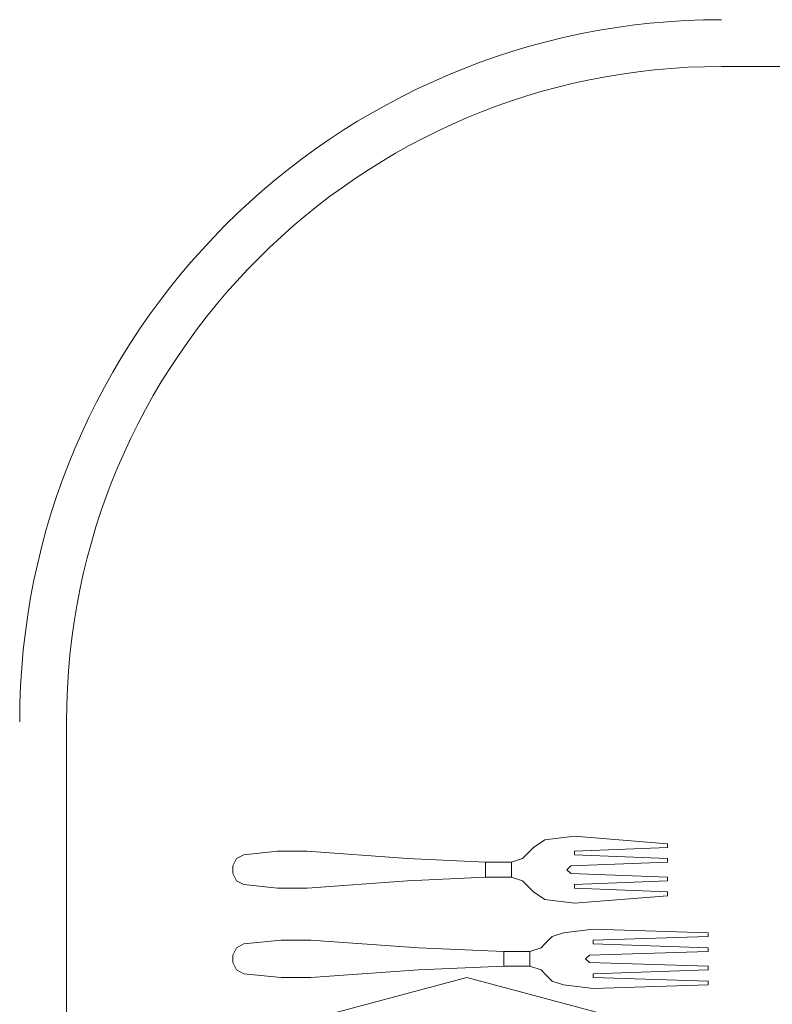
# Model space of a CAD drawing. Units: inches. Extents: x 375 to 1122, y 27 to 1069.
# Tile 125 of 155: x 705.14 to 717.62, y 900.21 to 916.52. Entities that reach past the tile are written whole.
import ezdxf

# ---------------------------------------------------------------- set-up
doc = ezdxf.new("R2010")
doc.units = ezdxf.units.IN
doc.layers.add('A-ANNO-DIMS', color=2, linetype='Continuous', lineweight=18)
doc.layers.add('Furniture', color=30, linetype='Continuous', lineweight=18)
doc.styles.get("Standard").update_dxf_attribs({"font": 'arial.ttf'})
doc.dimstyles.new('ISO-25', dxfattribs={"dimtxt": 12, "dimasz": 2.5, "dimexe": 1.5, "dimexo": 1.5, "dimtad": 1, "dimdec": 1, "dimlunit": 3, "dimtxsty": 'Standard', "dimblk": 'ARCHTICK', "dimcen": 2.5, "dimadec": 0, "dimazin": 0, "dimtfac": 1, "dimtdec": 1, "dimtmove": 0, "dimatfit": 3, "dimfxl": 1.5, "dimfxlon": 1, "dimarcsym": 0})

# ---------------------------------------------------------------- blocks, each defined once
blk = doc.blocks.new('A$C403C54AD')
for p, q in [((0.56427, 0.79569, -0.0006), (0.56427, 1.26108, -0.0006)), ((0.92321, 0.73013, -0.02105), (0.92475, 0.72551, -0.02059)), ((0.92321, 0.73013, -0.02413), (0.92475, 0.72551, -0.02367)), ((0.88473, 0.72244, -0.02105), (0.88781, 0.71782, -0.02059)), ((0.88473, 0.72244, -0.02413), (0.88781, 0.71782, -0.02367)), ((0.83575, 0.52421, -0.0006), (1.99923, 0.52421, -0.0006))]:
    blk.add_line(p, q)
for radius in [0.29087, 0.27148]:
    blk.add_arc((0.83575, 0.79569, -0.0006), radius, 180, 270)
for points, invisible_edges in [([(0.92629, 0.74244, -0.02045), (0.92167, 0.74244, -0.02045), (0.92321, 0.79016, -0.01335), (0.92475, 0.79016, -0.01335)], 1), ([(0.92629, 0.74244, -0.02353), (0.92167, 0.74244, -0.02353), (0.92321, 0.79016, -0.01643), (0.92475, 0.79016, -0.01643)], 1), ([(0.93244, 0.74091, -0.0207), (0.92782, 0.74244, -0.02045), (0.92936, 0.79016, -0.01335), (0.9309, 0.79016, -0.01335)], 1), ([(0.93244, 0.74091, -0.02378), (0.92782, 0.74244, -0.02353), (0.92936, 0.79016, -0.01643), (0.9309, 0.79016, -0.01643)], 1), ([(0.94014, 0.74244, -0.02045), (0.93552, 0.74091, -0.0207), (0.93706, 0.79016, -0.01335), (0.9386, 0.79016, -0.01335)], 1), ([(0.94014, 0.74244, -0.02353), (0.93552, 0.74091, -0.02378), (0.93706, 0.79016, -0.01643), (0.9386, 0.79016, -0.01643)], 1), ([(0.94168, 0.74244, -0.02045), (0.9463, 0.74244, -0.02045), (0.94476, 0.79016, -0.01335), (0.94322, 0.79016, -0.01335)], 1), ([(0.94168, 0.74244, -0.02353), (0.9463, 0.74244, -0.02353), (0.94476, 0.79016, -0.01643), (0.94322, 0.79016, -0.01643)], 1), ([(0.88935, 0.73475, -0.02045), (0.88319, 0.73475, -0.02045), (0.88627, 0.77323, -0.01335), (0.88781, 0.77323, -0.01335)], 1), ([(0.88935, 0.73475, -0.02353), (0.88319, 0.73475, -0.02353), (0.88627, 0.77323, -0.01643), (0.88781, 0.77323, -0.01643)], 1), ([(0.8955, 0.73321, -0.0207), (0.89088, 0.73475, -0.02045), (0.89242, 0.77323, -0.01335), (0.89396, 0.77323, -0.01335)], 1), ([(0.8955, 0.73321, -0.02378), (0.89088, 0.73475, -0.02353), (0.89242, 0.77323, -0.01643), (0.89396, 0.77323, -0.01643)], 1), ([(0.9032, 0.73475, -0.02045), (0.89858, 0.73321, -0.0207), (0.90012, 0.77323, -0.01335), (0.90166, 0.77323, -0.01335)], 1), ([(0.9032, 0.73475, -0.02353), (0.89858, 0.73321, -0.02378), (0.90012, 0.77323, -0.01643), (0.90166, 0.77323, -0.01643)], 1), ([(0.90474, 0.73475, -0.02045), (0.91089, 0.73475, -0.02045), (0.90782, 0.77323, -0.01335), (0.90628, 0.77323, -0.01335)], 1), ([(0.90474, 0.73475, -0.02353), (0.91089, 0.73475, -0.02353), (0.90782, 0.77323, -0.01643), (0.90628, 0.77323, -0.01643)], 1), ([(0.92321, 0.73013, -0.02105), (0.92782, 0.74244, -0.02045), (0.92629, 0.74244, -0.02045), (0.92167, 0.74244, -0.02045)], 5), ([(0.92321, 0.73013, -0.02413), (0.92782, 0.74244, -0.02353), (0.92629, 0.74244, -0.02353), (0.92167, 0.74244, -0.02353)], 5), ([(0.92321, 0.73013, -0.02413), (0.92321, 0.73013, -0.02105), (0.92167, 0.74244, -0.02045), (0.92167, 0.74244, -0.02353)], 1), ([(0.92321, 0.73013, -0.02105), (0.93398, 0.73924, -0.02085), (0.93244, 0.74091, -0.0207), (0.92782, 0.74244, -0.02045)], 13), ([(0.92321, 0.73013, -0.02413), (0.93398, 0.73924, -0.02392), (0.93244, 0.74091, -0.02378), (0.92782, 0.74244, -0.02353)], 13), ([(0.94476, 0.73013, -0.02105), (0.93398, 0.73924, -0.02085), (0.93552, 0.74091, -0.0207), (0.94014, 0.74244, -0.02045)], 13), ([(0.94476, 0.73013, -0.02413), (0.93398, 0.73924, -0.02392), (0.93552, 0.74091, -0.02378), (0.94014, 0.74244, -0.02353)], 13), ([(0.94476, 0.73013, -0.02105), (0.94014, 0.74244, -0.02045), (0.94168, 0.74244, -0.02045), (0.9463, 0.74244, -0.02045)], 5), ([(0.94476, 0.73013, -0.02413), (0.94014, 0.74244, -0.02353), (0.94168, 0.74244, -0.02353), (0.9463, 0.74244, -0.02353)], 5), ([(0.94476, 0.73013, -0.02105), (0.94476, 0.73013, -0.02413), (0.9463, 0.74244, -0.02353), (0.9463, 0.74244, -0.02045)], 1), ([(0.94476, 0.73013, -0.02105), (0.93398, 0.73924, -0.02085), (0.92321, 0.73013, -0.02105), (0.94476, 0.73013, -0.02105)], 7), ([(0.94476, 0.73013, -0.02413), (0.93398, 0.73924, -0.02392), (0.92321, 0.73013, -0.02413), (0.94476, 0.73013, -0.02413)], 7), ([(0.88473, 0.72244, -0.02105), (0.89088, 0.73475, -0.02045), (0.88935, 0.73475, -0.02045), (0.88319, 0.73475, -0.02045)], 5), ([(0.88473, 0.72244, -0.02413), (0.89088, 0.73475, -0.02353), (0.88935, 0.73475, -0.02353), (0.88319, 0.73475, -0.02353)], 5), ([(0.88473, 0.72244, -0.02413), (0.88473, 0.72244, -0.02105), (0.88319, 0.73475, -0.02045), (0.88319, 0.73475, -0.02353)], 1), ([(0.88473, 0.72244, -0.02105), (0.89704, 0.73155, -0.02085), (0.8955, 0.73321, -0.0207), (0.89088, 0.73475, -0.02045)], 13), ([(0.88473, 0.72244, -0.02413), (0.89704, 0.73155, -0.02392), (0.8955, 0.73321, -0.02378), (0.89088, 0.73475, -0.02353)], 13), ([(0.90935, 0.72244, -0.02105), (0.89704, 0.73155, -0.02085), (0.89858, 0.73321, -0.0207), (0.9032, 0.73475, -0.02045)], 13), ([(0.90935, 0.72244, -0.02413), (0.89704, 0.73155, -0.02392), (0.89858, 0.73321, -0.02378), (0.9032, 0.73475, -0.02353)], 13), ([(0.90935, 0.72244, -0.02105), (0.9032, 0.73475, -0.02045), (0.90474, 0.73475, -0.02045), (0.91089, 0.73475, -0.02045)], 5), ([(0.90935, 0.72244, -0.02413), (0.9032, 0.73475, -0.02353), (0.90474, 0.73475, -0.02353), (0.91089, 0.73475, -0.02353)], 5), ([(0.90935, 0.72244, -0.02105), (0.90935, 0.72244, -0.02413), (0.91089, 0.73475, -0.02353), (0.91089, 0.73475, -0.02045)], 1), ([(0.90935, 0.72244, -0.02105), (0.89704, 0.73155, -0.02085), (0.88473, 0.72244, -0.02105), (0.90935, 0.72244, -0.02105)], 7), ([(0.90935, 0.72244, -0.02413), (0.89704, 0.73155, -0.02392), (0.88473, 0.72244, -0.02413), (0.90935, 0.72244, -0.02413)], 7), ([(0.94322, 0.72551, -0.02059), (0.92475, 0.72551, -0.02059), (0.92321, 0.73013, -0.02105), (0.94476, 0.73013, -0.02105)], 5), ([(0.94322, 0.72551, -0.02367), (0.92475, 0.72551, -0.02367), (0.92321, 0.73013, -0.02413), (0.94476, 0.73013, -0.02413)], 5), ([(0.92475, 0.72551, -0.02059), (0.92475, 0.72551, -0.02367), (0.92321, 0.73013, -0.02413), (0.92321, 0.73013, -0.02105)], 4), ([(0.94322, 0.72551, -0.02367), (0.94322, 0.72551, -0.02059), (0.94476, 0.73013, -0.02105), (0.94476, 0.73013, -0.02413)], 4), ([(0.90628, 0.71782, -0.02059), (0.88781, 0.71782, -0.02059), (0.88473, 0.72244, -0.02105), (0.90935, 0.72244, -0.02105)], 5), ([(0.90628, 0.71782, -0.02367), (0.88781, 0.71782, -0.02367), (0.88473, 0.72244, -0.02413), (0.90935, 0.72244, -0.02413)], 5), ([(0.88781, 0.71782, -0.02059), (0.88781, 0.71782, -0.02367), (0.88473, 0.72244, -0.02413), (0.88473, 0.72244, -0.02105)], 4), ([(0.90628, 0.71782, -0.02367), (0.90628, 0.71782, -0.02059), (0.90935, 0.72244, -0.02105), (0.90935, 0.72244, -0.02413)], 4), ([(0.92782, 0.72244, -0.02243), (0.94014, 0.72244, -0.02243), (0.94322, 0.72551, -0.02367), (0.92475, 0.72551, -0.02367)], 5), ([(0.92782, 0.72244, -0.01935), (0.94014, 0.72244, -0.01935), (0.94322, 0.72551, -0.02059), (0.92475, 0.72551, -0.02059)], 5), ([(0.92936, 0.7209, -0.0183), (0.9386, 0.7209, -0.0183), (0.94014, 0.72244, -0.01935), (0.92782, 0.72244, -0.01935)], 5), ([(0.92936, 0.7209, -0.02109), (0.9386, 0.7209, -0.02109), (0.94014, 0.72244, -0.02243), (0.92782, 0.72244, -0.02243)], 5), ([(0.92936, 0.7209, -0.0183), (0.92936, 0.7209, -0.02109), (0.92782, 0.72244, -0.02243), (0.92782, 0.72244, -0.01935)], 1), ([(0.9386, 0.7209, -0.02109), (0.9386, 0.7209, -0.0183), (0.94014, 0.72244, -0.01935), (0.94014, 0.72244, -0.02243)], 1), ([(0.93706, 0.71628, -0.01595), (0.9309, 0.71628, -0.01595), (0.92936, 0.7209, -0.0183), (0.9386, 0.7209, -0.0183)], 4), ([(0.9309, 0.71628, -0.01854), (0.9309, 0.71628, -0.01595), (0.92936, 0.7209, -0.0183), (0.92936, 0.7209, -0.02109)], 5), ([(0.93706, 0.71628, -0.01854), (0.9309, 0.71628, -0.01854), (0.92936, 0.7209, -0.02109), (0.9386, 0.7209, -0.02109)], 4), ([(0.93706, 0.71628, -0.01595), (0.93706, 0.71628, -0.01854), (0.9386, 0.7209, -0.02109), (0.9386, 0.7209, -0.0183)], 5), ([(0.89088, 0.71474, -0.02243), (0.9032, 0.71474, -0.02243), (0.90628, 0.71782, -0.02367), (0.88781, 0.71782, -0.02367)], 5), ([(0.89088, 0.71474, -0.01935), (0.9032, 0.71474, -0.01935), (0.90628, 0.71782, -0.02059), (0.88781, 0.71782, -0.02059)], 5), ([(0.89242, 0.7132, -0.0183), (0.90166, 0.7132, -0.0183), (0.9032, 0.71474, -0.01935), (0.89088, 0.71474, -0.01935)], 5), ([(0.89242, 0.7132, -0.02109), (0.90166, 0.7132, -0.02109), (0.9032, 0.71474, -0.02243), (0.89088, 0.71474, -0.02243)], 5), ([(0.89242, 0.7132, -0.0183), (0.89242, 0.7132, -0.02109), (0.89088, 0.71474, -0.02243), (0.89088, 0.71474, -0.01935)], 1), ([(0.90166, 0.7132, -0.02109), (0.90166, 0.7132, -0.0183), (0.9032, 0.71474, -0.01935), (0.9032, 0.71474, -0.02243)], 1), ([(0.9309, 0.71628, -0.01854), (0.9309, 0.71628, -0.01595), (0.9309, 0.7055, -0.01387), (0.9309, 0.7055, -0.01646)], 5), ([(0.93706, 0.7055, -0.01646), (0.93706, 0.7055, -0.01387), (0.93706, 0.71628, -0.01595), (0.93706, 0.71628, -0.01854)], 5), ([(0.90012, 0.70858, -0.01595), (0.89396, 0.70858, -0.01595), (0.89242, 0.7132, -0.0183), (0.90166, 0.7132, -0.0183)], 4), ([(0.90012, 0.70858, -0.01854), (0.89396, 0.70858, -0.01854), (0.89242, 0.7132, -0.02109), (0.90166, 0.7132, -0.02109)], 4), ([(0.89396, 0.70858, -0.01854), (0.89396, 0.70858, -0.01595), (0.89242, 0.7132, -0.0183), (0.89242, 0.7132, -0.02109)], 5), ([(0.90012, 0.70858, -0.01595), (0.90012, 0.70858, -0.01854), (0.90166, 0.7132, -0.02109), (0.90166, 0.7132, -0.0183)], 5), ([(0.89396, 0.70858, -0.01854), (0.89396, 0.70858, -0.01595), (0.89396, 0.69781, -0.01387), (0.89396, 0.69781, -0.01646)], 5), ([(0.90012, 0.69781, -0.01646), (0.90012, 0.69781, -0.01387), (0.90012, 0.70858, -0.01595), (0.90012, 0.70858, -0.01854)], 5), ([(0.9386, 0.6701, -0.01678), (0.92936, 0.6701, -0.01678), (0.9309, 0.7055, -0.01387), (0.93706, 0.7055, -0.01387)], 1), ([(0.9309, 0.7055, -0.01387), (0.9309, 0.7055, -0.01646), (0.92936, 0.6701, -0.01986), (0.92936, 0.6701, -0.01678)], 5), ([(0.9386, 0.6701, -0.01986), (0.92936, 0.6701, -0.01986), (0.9309, 0.7055, -0.01646), (0.93706, 0.7055, -0.01646)], 1), ([(0.9386, 0.6701, -0.01678), (0.9386, 0.6701, -0.01986), (0.93706, 0.7055, -0.01646), (0.93706, 0.7055, -0.01387)], 5), ([(0.90166, 0.66549, -0.01678), (0.89242, 0.66549, -0.01678), (0.89396, 0.69781, -0.01387), (0.90012, 0.69781, -0.01387)], 1), ([(0.89396, 0.69781, -0.01387), (0.89396, 0.69781, -0.01646), (0.89242, 0.66549, -0.01986), (0.89242, 0.66549, -0.01678)], 5), ([(0.90166, 0.66549, -0.01986), (0.89242, 0.66549, -0.01986), (0.89396, 0.69781, -0.01646), (0.90012, 0.69781, -0.01646)], 1), ([(0.90166, 0.66549, -0.01678), (0.90166, 0.66549, -0.01986), (0.90012, 0.69781, -0.01646), (0.90012, 0.69781, -0.01387)], 5), ([(0.92629, 0.62547, -0.01916), (0.94168, 0.62547, -0.01916), (0.9386, 0.6701, -0.01678), (0.92936, 0.6701, -0.01678)], 5), ([(0.92629, 0.62547, -0.0238), (0.94168, 0.62547, -0.0238), (0.9386, 0.6701, -0.01986), (0.92936, 0.6701, -0.01986)], 5), ([(0.92936, 0.6701, -0.01986), (0.92936, 0.6701, -0.01678), (0.92629, 0.62547, -0.01916), (0.92629, 0.62547, -0.0238)], 1), ([(0.94168, 0.62547, -0.0238), (0.94168, 0.62547, -0.01916), (0.9386, 0.6701, -0.01678), (0.9386, 0.6701, -0.01986)], 4), ([(0.88935, 0.62393, -0.01916), (0.90474, 0.62393, -0.01916), (0.90166, 0.66549, -0.01678), (0.89242, 0.66549, -0.01678)], 5), ([(0.88935, 0.62393, -0.0238), (0.90474, 0.62393, -0.0238), (0.90166, 0.66549, -0.01986), (0.89242, 0.66549, -0.01986)], 5), ([(0.89242, 0.66549, -0.01986), (0.89242, 0.66549, -0.01678), (0.88935, 0.62393, -0.01916), (0.88935, 0.62393, -0.0238)], 1), ([(0.90474, 0.62393, -0.0238), (0.90474, 0.62393, -0.01916), (0.90166, 0.66549, -0.01678), (0.90166, 0.66549, -0.01986)], 4), ([(0.94168, 0.61315, -0.01949), (0.92629, 0.61315, -0.01949), (0.92629, 0.62547, -0.01916), (0.94168, 0.62547, -0.01916)], 5), ([(0.94168, 0.61315, -0.02413), (0.92629, 0.61315, -0.02413), (0.92629, 0.62547, -0.0238), (0.94168, 0.62547, -0.0238)], 5), ([(0.90474, 0.61161, -0.01949), (0.88935, 0.61161, -0.01949), (0.88935, 0.62393, -0.01916), (0.90474, 0.62393, -0.01916)], 5), ([(0.90474, 0.61161, -0.02413), (0.88935, 0.61161, -0.02413), (0.88935, 0.62393, -0.0238), (0.90474, 0.62393, -0.0238)], 5), ([(0.92782, 0.59776, -0.01946), (0.94014, 0.59776, -0.01946), (0.94168, 0.61315, -0.01949), (0.92629, 0.61315, -0.01949)], 5), ([(0.92782, 0.59776, -0.02409), (0.94014, 0.59776, -0.02409), (0.94168, 0.61315, -0.02413), (0.92629, 0.61315, -0.02413)], 5), ([(0.89088, 0.59776, -0.01946), (0.9032, 0.59776, -0.01946), (0.90474, 0.61161, -0.01949), (0.88935, 0.61161, -0.01949)], 5), ([(0.89088, 0.59776, -0.02409), (0.9032, 0.59776, -0.02409), (0.90474, 0.61161, -0.02413), (0.88935, 0.61161, -0.02413)], 5), ([(0.90166, 0.59468, -0.01921), (0.89242, 0.59468, -0.01921), (0.89088, 0.59776, -0.01946), (0.9032, 0.59776, -0.01946)], 5), ([(0.90166, 0.59468, -0.02385), (0.89242, 0.59468, -0.02385), (0.89088, 0.59776, -0.02409), (0.9032, 0.59776, -0.02409)], 5), ([(0.9386, 0.59468, -0.01921), (0.92936, 0.59468, -0.01921), (0.92782, 0.59776, -0.01946), (0.94014, 0.59776, -0.01946)], 5), ([(0.9386, 0.59468, -0.02385), (0.92936, 0.59468, -0.02385), (0.92782, 0.59776, -0.02409), (0.94014, 0.59776, -0.02409)], 5), ([(0.8955, 0.59314, -0.01938), (0.89858, 0.59314, -0.01938), (0.90166, 0.59468, -0.01921), (0.89242, 0.59468, -0.01921)], 4), ([(0.8955, 0.59314, -0.02351), (0.89858, 0.59314, -0.02351), (0.90166, 0.59468, -0.02385), (0.89242, 0.59468, -0.02385)], 4), ([(0.93244, 0.59314, -0.01938), (0.93552, 0.59314, -0.01938), (0.9386, 0.59468, -0.01921), (0.92936, 0.59468, -0.01921)], 4), ([(0.93244, 0.59314, -0.02351), (0.93552, 0.59314, -0.02351), (0.9386, 0.59468, -0.02385), (0.92936, 0.59468, -0.02385)], 4)]:
    blk.add_3dface(points, dxfattribs=dict(invisible_edges=invisible_edges))
for points in [[(0.92321, 0.79016, -0.01335), (0.92321, 0.79016, -0.01643), (0.92167, 0.74244, -0.02353), (0.92167, 0.74244, -0.02045)], [(0.92475, 0.79016, -0.01643), (0.92475, 0.79016, -0.01335), (0.92321, 0.79016, -0.01335), (0.92321, 0.79016, -0.01643)], [(0.92629, 0.74244, -0.02045), (0.92629, 0.74244, -0.02353), (0.92475, 0.79016, -0.01643), (0.92475, 0.79016, -0.01335)], [(0.92936, 0.79016, -0.01335), (0.92936, 0.79016, -0.01643), (0.92782, 0.74244, -0.02353), (0.92782, 0.74244, -0.02045)], [(0.9309, 0.79016, -0.01643), (0.9309, 0.79016, -0.01335), (0.92936, 0.79016, -0.01335), (0.92936, 0.79016, -0.01643)], [(0.93244, 0.74091, -0.02378), (0.93244, 0.74091, -0.0207), (0.9309, 0.79016, -0.01335), (0.9309, 0.79016, -0.01643)], [(0.93706, 0.79016, -0.01643), (0.93706, 0.79016, -0.01335), (0.93552, 0.74091, -0.0207), (0.93552, 0.74091, -0.02378)], [(0.9386, 0.79016, -0.01643), (0.9386, 0.79016, -0.01335), (0.93706, 0.79016, -0.01335), (0.93706, 0.79016, -0.01643)], [(0.94014, 0.74244, -0.02353), (0.94014, 0.74244, -0.02045), (0.9386, 0.79016, -0.01335), (0.9386, 0.79016, -0.01643)], [(0.94322, 0.79016, -0.01335), (0.94322, 0.79016, -0.01643), (0.94168, 0.74244, -0.02353), (0.94168, 0.74244, -0.02045)], [(0.94476, 0.79016, -0.01643), (0.94476, 0.79016, -0.01335), (0.94322, 0.79016, -0.01335), (0.94322, 0.79016, -0.01643)], [(0.9463, 0.74244, -0.02353), (0.9463, 0.74244, -0.02045), (0.94476, 0.79016, -0.01335), (0.94476, 0.79016, -0.01643)], [(0.88627, 0.77323, -0.01335), (0.88627, 0.77323, -0.01643), (0.88319, 0.73475, -0.02353), (0.88319, 0.73475, -0.02045)], [(0.88781, 0.77323, -0.01643), (0.88781, 0.77323, -0.01335), (0.88627, 0.77323, -0.01335), (0.88627, 0.77323, -0.01643)], [(0.88935, 0.73475, -0.02045), (0.88935, 0.73475, -0.02353), (0.88781, 0.77323, -0.01643), (0.88781, 0.77323, -0.01335)], [(0.89242, 0.77323, -0.01335), (0.89242, 0.77323, -0.01643), (0.89088, 0.73475, -0.02353), (0.89088, 0.73475, -0.02045)], [(0.89396, 0.77323, -0.01643), (0.89396, 0.77323, -0.01335), (0.89242, 0.77323, -0.01335), (0.89242, 0.77323, -0.01643)], [(0.8955, 0.73321, -0.02378), (0.8955, 0.73321, -0.0207), (0.89396, 0.77323, -0.01335), (0.89396, 0.77323, -0.01643)], [(0.90012, 0.77323, -0.01643), (0.90012, 0.77323, -0.01335), (0.89858, 0.73321, -0.0207), (0.89858, 0.73321, -0.02378)], [(0.90166, 0.77323, -0.01643), (0.90166, 0.77323, -0.01335), (0.90012, 0.77323, -0.01335), (0.90012, 0.77323, -0.01643)], [(0.9032, 0.73475, -0.02353), (0.9032, 0.73475, -0.02045), (0.90166, 0.77323, -0.01335), (0.90166, 0.77323, -0.01643)], [(0.90628, 0.77323, -0.01335), (0.90628, 0.77323, -0.01643), (0.90474, 0.73475, -0.02353), (0.90474, 0.73475, -0.02045)], [(0.90782, 0.77323, -0.01643), (0.90782, 0.77323, -0.01335), (0.90628, 0.77323, -0.01335), (0.90628, 0.77323, -0.01643)], [(0.91089, 0.73475, -0.02353), (0.91089, 0.73475, -0.02045), (0.90782, 0.77323, -0.01335), (0.90782, 0.77323, -0.01643)], [(0.92629, 0.74244, -0.02045), (0.92629, 0.74244, -0.02353), (0.92782, 0.74244, -0.02353), (0.92782, 0.74244, -0.02045)], [(0.94014, 0.74244, -0.02353), (0.94014, 0.74244, -0.02045), (0.94168, 0.74244, -0.02045), (0.94168, 0.74244, -0.02353)], [(0.93244, 0.74091, -0.0207), (0.93244, 0.74091, -0.02378), (0.93398, 0.73924, -0.02392), (0.93398, 0.73924, -0.02085)], [(0.93398, 0.73924, -0.02392), (0.93398, 0.73924, -0.02085), (0.93552, 0.74091, -0.0207), (0.93552, 0.74091, -0.02378)], [(0.88935, 0.73475, -0.02045), (0.88935, 0.73475, -0.02353), (0.89088, 0.73475, -0.02353), (0.89088, 0.73475, -0.02045)], [(0.9032, 0.73475, -0.02353), (0.9032, 0.73475, -0.02045), (0.90474, 0.73475, -0.02045), (0.90474, 0.73475, -0.02353)], [(0.8955, 0.73321, -0.0207), (0.8955, 0.73321, -0.02378), (0.89704, 0.73155, -0.02392), (0.89704, 0.73155, -0.02085)], [(0.89704, 0.73155, -0.02392), (0.89704, 0.73155, -0.02085), (0.89858, 0.73321, -0.0207), (0.89858, 0.73321, -0.02378)], [(0.92782, 0.72244, -0.02243), (0.92782, 0.72244, -0.01935), (0.92475, 0.72551, -0.02059), (0.92475, 0.72551, -0.02367)], [(0.94014, 0.72244, -0.01935), (0.94014, 0.72244, -0.02243), (0.94322, 0.72551, -0.02367), (0.94322, 0.72551, -0.02059)], [(0.89088, 0.71474, -0.02243), (0.89088, 0.71474, -0.01935), (0.88781, 0.71782, -0.02059), (0.88781, 0.71782, -0.02367)], [(0.9032, 0.71474, -0.01935), (0.9032, 0.71474, -0.02243), (0.90628, 0.71782, -0.02367), (0.90628, 0.71782, -0.02059)], [(0.9309, 0.7055, -0.01387), (0.93706, 0.7055, -0.01387), (0.93706, 0.71628, -0.01595), (0.9309, 0.71628, -0.01595)], [(0.9309, 0.7055, -0.01646), (0.93706, 0.7055, -0.01646), (0.93706, 0.71628, -0.01854), (0.9309, 0.71628, -0.01854)], [(0.89396, 0.69781, -0.01387), (0.90012, 0.69781, -0.01387), (0.90012, 0.70858, -0.01595), (0.89396, 0.70858, -0.01595)], [(0.89396, 0.69781, -0.01646), (0.90012, 0.69781, -0.01646), (0.90012, 0.70858, -0.01854), (0.89396, 0.70858, -0.01854)], [(0.92629, 0.62547, -0.01916), (0.92629, 0.62547, -0.0238), (0.92629, 0.61315, -0.02413), (0.92629, 0.61315, -0.01949)], [(0.94168, 0.61315, -0.01949), (0.94168, 0.61315, -0.02413), (0.94168, 0.62547, -0.0238), (0.94168, 0.62547, -0.01916)], [(0.88935, 0.62393, -0.01916), (0.88935, 0.62393, -0.0238), (0.88935, 0.61161, -0.02413), (0.88935, 0.61161, -0.01949)], [(0.90474, 0.61161, -0.01949), (0.90474, 0.61161, -0.02413), (0.90474, 0.62393, -0.0238), (0.90474, 0.62393, -0.01916)], [(0.92629, 0.61315, -0.02413), (0.92629, 0.61315, -0.01949), (0.92782, 0.59776, -0.01946), (0.92782, 0.59776, -0.02409)], [(0.94014, 0.59776, -0.02409), (0.94014, 0.59776, -0.01946), (0.94168, 0.61315, -0.01949), (0.94168, 0.61315, -0.02413)], [(0.88935, 0.61161, -0.02413), (0.88935, 0.61161, -0.01949), (0.89088, 0.59776, -0.01946), (0.89088, 0.59776, -0.02409)], [(0.9032, 0.59776, -0.02409), (0.9032, 0.59776, -0.01946), (0.90474, 0.61161, -0.01949), (0.90474, 0.61161, -0.02413)], [(0.89088, 0.59776, -0.01946), (0.89088, 0.59776, -0.02409), (0.89242, 0.59468, -0.02385), (0.89242, 0.59468, -0.01921)], [(0.90166, 0.59468, -0.01921), (0.90166, 0.59468, -0.02385), (0.9032, 0.59776, -0.02409), (0.9032, 0.59776, -0.01946)], [(0.92782, 0.59776, -0.01946), (0.92782, 0.59776, -0.02409), (0.92936, 0.59468, -0.02385), (0.92936, 0.59468, -0.01921)], [(0.9386, 0.59468, -0.01921), (0.9386, 0.59468, -0.02385), (0.94014, 0.59776, -0.02409), (0.94014, 0.59776, -0.01946)], [(0.89242, 0.59468, -0.02385), (0.89242, 0.59468, -0.01921), (0.8955, 0.59314, -0.01938), (0.8955, 0.59314, -0.02351)], [(0.8955, 0.59314, -0.01938), (0.8955, 0.59314, -0.02351), (0.89858, 0.59314, -0.02351), (0.89858, 0.59314, -0.01938)], [(0.89858, 0.59314, -0.02351), (0.89858, 0.59314, -0.01938), (0.90166, 0.59468, -0.01921), (0.90166, 0.59468, -0.02385)], [(0.92936, 0.59468, -0.02385), (0.92936, 0.59468, -0.01921), (0.93244, 0.59314, -0.01938), (0.93244, 0.59314, -0.02351)], [(0.93244, 0.59314, -0.01938), (0.93244, 0.59314, -0.02351), (0.93552, 0.59314, -0.02351), (0.93552, 0.59314, -0.01938)], [(0.93552, 0.59314, -0.02351), (0.93552, 0.59314, -0.01938), (0.9386, 0.59468, -0.01921), (0.9386, 0.59468, -0.02385)]]:
    blk.add_3dface(points)
at = {"linetype": 'ByBlock', "invisible_edges": 5}
for points in [[(0.96024, 0.75938, -0.00874), (0.97623, 0.75014, -0.00874), (0.96015, 0.69011, -0.00874), (0.94168, 0.69011, -0.00874)], [(0.98956, 0.74244, -0.02259), (0.96024, 0.75938, -0.01335), (0.94168, 0.69011, -0.01335), (0.97554, 0.69011, -0.02259)], [(0.94168, 0.69011, -0.00874), (0.96015, 0.69011, -0.00874), (0.97623, 0.63008, -0.00874), (0.96024, 0.62085, -0.00874)], [(0.97554, 0.69011, -0.02259), (0.94168, 0.69011, -0.01335), (0.96024, 0.62085, -0.01335), (0.98956, 0.63778, -0.02259)]]:
    blk.add_3dface(points, dxfattribs=at)
at = {"linetype": 'ByBlock'}
for points in [[(0.96024, 0.75938, -0.01335), (0.96024, 0.75938, -0.00874), (0.94168, 0.69011, -0.00874), (0.94168, 0.69011, -0.01335)], [(0.94168, 0.69011, -0.01335), (0.94168, 0.69011, -0.00874), (0.96024, 0.62085, -0.00874), (0.96024, 0.62085, -0.01335)]]:
    blk.add_3dface(points, dxfattribs=at)
blk = doc.blocks.new('_ArchTick')
at = {"color": 0, "linetype": 'ByBlock', "const_width": 0.15}
blk.add_lwpolyline([(-0.5, -0.5), (0.5, 0.5)], dxfattribs=at)
blk = doc.blocks.new('*D73')
at = {"layer": 'A-ANNO-DIMS', "color": 0, "lineweight": -2, "transparency": 16777216}
for p, q in [((686.757, 932.428), (686.757, 929.428)), ((770.757, 932.428), (770.757, 929.428)), ((686.757, 930.928), (770.757, 930.928)), ((770.757, 930.928), (987.61, 930.928))]:
    blk.add_line(p, q, dxfattribs=at)
at = {"layer": 'Defpoints', "color": 0, "transparency": 16777216}
for p in [(686.757, 943.528), (770.757, 943.528), (770.757, 930.928)]:
    blk.add_point(p, dxfattribs=at)
at = {"layer": 'A-ANNO-DIMS', "color": 0, "lineweight": -2, "transparency": 16777216, "xscale": 2.5, "yscale": 2.5, "zscale": 2.5, "rotation": 180}
blk.add_blockref('_ArchTick', (686.757, 930.928), dxfattribs=at)
at = {"layer": 'A-ANNO-DIMS', "color": 0, "lineweight": -2, "transparency": 16777216, "xscale": 2.5, "yscale": 2.5, "zscale": 2.5}
blk.add_blockref('_ArchTick', (770.757, 930.928), dxfattribs=at)
at = {"layer": 'A-ANNO-DIMS', "color": 0, "transparency": 16777216, "insert": (880.433, 937.757), "char_height": 12, "attachment_point": 5}
blk.add_mtext('2-PANEL SLIDER 7\'-0" TYP.', dxfattribs=at)

msp = doc.modelspace()

# ---------------------------------------------------------------- block references
at = {"layer": 'Furniture', "xscale": 39.9918517141215, "yscale": 39.9918517141215, "zscale": 39.9918517141215, "rotation": 270}
msp.add_blockref('A$C403C54AD', (684.955, 938.316, 0.024), dxfattribs=at)

# ---------------------------------------------------------------- dimensions: what is measured, and where the dimension line sits
at = {"layer": 'A-ANNO-DIMS'}
dim = msp.add_linear_dim(base=(770.757, 930.928), p1=(686.757, 943.528), p2=(770.757, 943.528), text='2-PANEL SLIDER <> TYP.', dimstyle='ISO-25', override={"dimdec": 1, "dimlfac": 1, "dimrnd": 0, "dimzin": 1, "dimdsep": 46, "dimlunit": 4, "dimfrac": 2}, dxfattribs=at)
dim.commit()
dim.dimension.update_dxf_attribs({"geometry": '*D73', "text_midpoint": (880.433, 937.757)})

doc.saveas('drawing.dxf')
